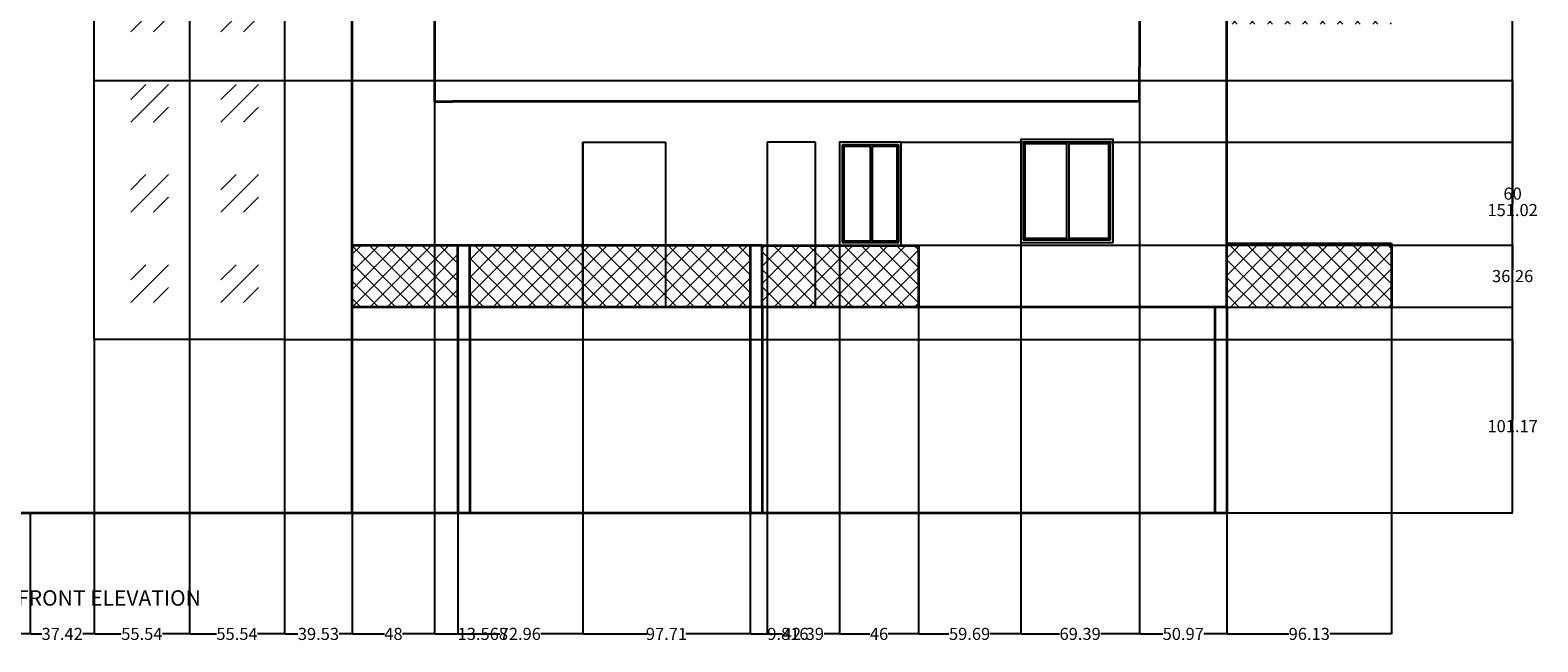
# Model space of a CAD drawing. Units: inches. Extents: x -222 to 1347, y 12 to 1073.
# Tile 3 of 4: x 467 to 1347, y 12 to 369. Entities that reach past the tile are written whole.
import ezdxf

# ---------------------------------------------------------------- set-up
doc = ezdxf.new("R2010")
doc.units = ezdxf.units.IN
doc.header["$MEASUREMENT"] = 0
for name, color, linetype, lineweight in [('A-ANNO-DIMS', 2, 'Continuous', 18), ('A-ANNO-TEXT', 7, 'Continuous', 25), ('A-DOOR', 4, 'Continuous', 25), ('A-ELEV', 7, 'Continuous', 35), ('A-ELEV-PATT', 8, 'Continuous', 13), ('A-GLAZ', 4, 'Continuous', 25)]:
    doc.layers.add(name, color=color, linetype=linetype, lineweight=lineweight)
doc.styles.get("Standard").update_dxf_attribs({"font": 'arial.ttf'})
doc.dimstyles.get("Standard").update_dxf_attribs({"dimtxt": 7.0625, "dimasz": 0.18, "dimexe": 0.18, "dimexo": 0.0625, "dimgap": 0.09, "dimtad": 0, "dimtih": 1, "dimtoh": 1, "dimdec": 4, "dimzin": 0, "dimdsep": 46, "dimlunit": 4, "dimtxsty": 'Standard', "dimcen": 0.09, "dimadec": 0, "dimazin": 0, "dimtfac": 1, "dimtdec": 4, "dimtofl": 0, "dimtmove": 0, "dimatfit": 3, "dimfxl": 1, "dimtolj": 1, "dimtzin": 0, "dimarcsym": 0})
pattern_1 = [(45, (-188.0434, -1e-13), (-5.126524, 5.126524), []), (135, (-188.0434, -1e-13), (-5.126524, -5.126524), [])]

# ---------------------------------------------------------------- blocks, each defined once
blk = doc.blocks.new('*U2')
for p, q in [((1.5, 1.5), (1.5, 58.5)), ((1.5, 58.5), (27, 58.5)), ((27, 1.5), (27, 58.5)), ((27, 58.5), (52.5, 58.5)), ((52.5, 58.5), (52.5, 1.5)), ((27, 1.5), (1.5, 1.5)), ((52.5, 1.5), (27, 1.5))]:
    blk.add_line(p, q)
blk.add_lwpolyline([(0, 0), (0, 60), (54, 60), (54, 0)], close=True)
for points in [[(26, 57.5), (26, 2.5), (2.5, 2.5), (2.5, 57.5), (26, 57.5)], [(27, 57.5), (51.5, 57.5), (51.5, 2.5), (27, 2.5)]]:
    blk.add_lwpolyline(points)
blk = doc.blocks.new('*U3')
for p, q in [((1.5, 1.5), (1.5, 58.5)), ((1.5, 58.5), (18, 58.5)), ((18, 1.5), (18, 58.5)), ((18, 58.5), (34.5, 58.5)), ((34.5, 58.5), (34.5, 1.5)), ((18, 1.5), (1.5, 1.5)), ((34.5, 1.5), (18, 1.5))]:
    blk.add_line(p, q)
blk.add_lwpolyline([(0, 0), (0, 60), (36, 60), (36, 0)], close=True)
for points in [[(17, 57.5), (17, 2.5), (2.5, 2.5), (2.5, 57.5), (17, 57.5)], [(18, 57.5), (33.5, 57.5), (33.5, 2.5), (18, 2.5)]]:
    blk.add_lwpolyline(points)
blk = doc.blocks.new('DOOR-700')
for p, q in [((0, 96.26), (0, 0)), ((0, 96.26), (23.43, 96.26)), ((23.43, 96.26), (28.14, 96.26)), ((28.14, 96.26), (28.14, 0))]:
    blk.add_line(p, q)
blk = doc.blocks.new('DOOR-1200')
for p, q in [((0, 0), (0, 96.26)), ((0, 96.26), (48.21, 96.26)), ((48.21, 96.26), (48.21, 0))]:
    blk.add_line(p, q)
blk = doc.blocks.new('*D21')
at = {"layer": 'A-ANNO-DIMS', "color": 0, "lineweight": -2, "transparency": 16777216}
for p, q in [((419.34, 327.6), (419.34, 16.83)), ((467.34, 87.6), (467.34, 16.83)), ((419.52, 17.01), (438.05, 17.01)), ((467.16, 17.01), (448.64, 17.01))]:
    blk.add_line(p, q, dxfattribs=at)
at = {"layer": 'A-ANNO-DIMS', "color": 0, "transparency": 16777216}
for points in [[(419.52, 17.04), (419.52, 16.98), (419.34, 17.01)], [(467.16, 17.04), (467.16, 16.98), (467.34, 17.01)]]:
    blk.add_solid(points, dxfattribs=at)
at = {"layer": 'Defpoints', "color": 0, "transparency": 16777216}
for p in [(419.34, 327.66), (467.34, 87.66), (467.34, 17.01)]:
    blk.add_point(p, dxfattribs=at)
at = {"layer": 'A-ANNO-DIMS', "color": 0, "transparency": 16777216, "insert": (443.34, 17.01), "char_height": 7.062, "attachment_point": 5}
blk.add_mtext('\\A1;48', dxfattribs=at)
blk = doc.blocks.new('*D22')
at = {"layer": 'A-ANNO-DIMS', "color": 0, "lineweight": -2, "transparency": 16777216}
for p, q in [((504.77, 188.77), (504.77, 16.83)), ((467.34, 87.6), (467.34, 16.83)), ((467.52, 17.01), (474.09, 17.01)), ((504.59, 17.01), (498.02, 17.01))]:
    blk.add_line(p, q, dxfattribs=at)
at = {"layer": 'A-ANNO-DIMS', "color": 0, "transparency": 16777216}
for points in [[(467.52, 17.04), (467.52, 16.98), (467.34, 17.01)], [(504.59, 17.04), (504.59, 16.98), (504.77, 17.01)]]:
    blk.add_solid(points, dxfattribs=at)
at = {"layer": 'Defpoints', "color": 0, "transparency": 16777216}
for p in [(504.77, 188.83), (467.34, 87.66), (504.77, 17.01)]:
    blk.add_point(p, dxfattribs=at)
at = {"layer": 'A-ANNO-DIMS', "color": 0, "transparency": 16777216, "insert": (486.05, 17.01), "char_height": 7.062, "attachment_point": 5}
blk.add_mtext('\\A1;37.42', dxfattribs=at)
blk = doc.blocks.new('*D23')
at = {"layer": 'A-ANNO-DIMS', "color": 0, "lineweight": -2, "transparency": 16777216}
for p, q in [((504.77, 188.77), (504.77, 16.83)), ((560.31, 188.77), (560.31, 16.83)), ((504.95, 17.01), (520.55, 17.01)), ((560.13, 17.01), (544.53, 17.01))]:
    blk.add_line(p, q, dxfattribs=at)
at = {"layer": 'A-ANNO-DIMS', "color": 0, "transparency": 16777216}
for points in [[(504.95, 17.04), (504.95, 16.98), (504.77, 17.01)], [(560.13, 17.04), (560.13, 16.98), (560.31, 17.01)]]:
    blk.add_solid(points, dxfattribs=at)
at = {"layer": 'Defpoints', "color": 0, "transparency": 16777216}
for p in [(504.77, 188.83), (560.31, 188.83), (560.31, 17.01)]:
    blk.add_point(p, dxfattribs=at)
at = {"layer": 'A-ANNO-DIMS', "color": 0, "transparency": 16777216, "insert": (532.54, 17.01), "char_height": 7.062, "attachment_point": 5}
blk.add_mtext('\\A1;55.54', dxfattribs=at)
blk = doc.blocks.new('*D24')
at = {"layer": 'A-ANNO-DIMS', "color": 0, "lineweight": -2, "transparency": 16777216}
for p, q in [((560.31, 188.77), (560.31, 16.83)), ((615.85, 188.77), (615.85, 16.83)), ((560.49, 17.01), (576.09, 17.01)), ((615.67, 17.01), (600.07, 17.01))]:
    blk.add_line(p, q, dxfattribs=at)
at = {"layer": 'A-ANNO-DIMS', "color": 0, "transparency": 16777216}
for points in [[(560.49, 17.04), (560.49, 16.98), (560.31, 17.01)], [(615.67, 17.04), (615.67, 16.98), (615.85, 17.01)]]:
    blk.add_solid(points, dxfattribs=at)
at = {"layer": 'Defpoints', "color": 0, "transparency": 16777216}
for p in [(560.31, 188.83), (615.85, 188.83), (615.85, 17.01)]:
    blk.add_point(p, dxfattribs=at)
at = {"layer": 'A-ANNO-DIMS', "color": 0, "transparency": 16777216, "insert": (588.08, 17.01), "char_height": 7.062, "attachment_point": 5}
blk.add_mtext('\\A1;55.54', dxfattribs=at)
blk = doc.blocks.new('*D25')
at = {"layer": 'A-ANNO-DIMS', "color": 0, "lineweight": -2, "transparency": 16777216}
for p, q in [((615.85, 188.77), (615.85, 16.83)), ((655.39, 87.6), (655.39, 16.83)), ((616.03, 17.01), (623.62, 17.01)), ((655.21, 17.01), (647.62, 17.01))]:
    blk.add_line(p, q, dxfattribs=at)
at = {"layer": 'A-ANNO-DIMS', "color": 0, "transparency": 16777216}
for points in [[(616.03, 17.04), (616.03, 16.98), (615.85, 17.01)], [(655.21, 17.04), (655.21, 16.98), (655.39, 17.01)]]:
    blk.add_solid(points, dxfattribs=at)
at = {"layer": 'Defpoints', "color": 0, "transparency": 16777216}
for p in [(615.85, 188.83), (655.39, 87.66), (655.39, 17.01)]:
    blk.add_point(p, dxfattribs=at)
at = {"layer": 'A-ANNO-DIMS', "color": 0, "transparency": 16777216, "insert": (635.62, 17.01), "char_height": 7.062, "attachment_point": 5}
blk.add_mtext('\\A1;39.53', dxfattribs=at)
blk = doc.blocks.new('*D26')
at = {"layer": 'A-ANNO-DIMS', "color": 0, "lineweight": -2, "transparency": 16777216}
for p, q in [((703.39, 327.6), (703.39, 16.83)), ((655.39, 87.6), (655.39, 16.83)), ((655.57, 17.01), (674.09, 17.01)), ((703.21, 17.01), (684.68, 17.01))]:
    blk.add_line(p, q, dxfattribs=at)
at = {"layer": 'A-ANNO-DIMS', "color": 0, "transparency": 16777216}
for points in [[(655.57, 17.04), (655.57, 16.98), (655.39, 17.01)], [(703.21, 17.04), (703.21, 16.98), (703.39, 17.01)]]:
    blk.add_solid(points, dxfattribs=at)
at = {"layer": 'Defpoints', "color": 0, "transparency": 16777216}
for p in [(703.39, 327.66), (655.39, 87.66), (703.39, 17.01)]:
    blk.add_point(p, dxfattribs=at)
at = {"layer": 'A-ANNO-DIMS', "color": 0, "transparency": 16777216, "insert": (679.39, 17.01), "char_height": 7.062, "attachment_point": 5}
blk.add_mtext('\\A1;48', dxfattribs=at)
blk = doc.blocks.new('*D27')
at = {"layer": 'A-ANNO-DIMS', "color": 0, "lineweight": -2, "transparency": 16777216}
for p, q in [((703.39, 327.6), (703.39, 16.83)), ((716.95, 87.6), (716.95, 16.83)), ((703.57, 17.01), (716.77, 17.01)), ((716.95, 17.01), (717.13, 17.01))]:
    blk.add_line(p, q, dxfattribs=at)
at = {"layer": 'A-ANNO-DIMS', "color": 0, "transparency": 16777216}
for points in [[(703.57, 17.04), (703.57, 16.98), (703.39, 17.01)], [(716.77, 17.04), (716.77, 16.98), (716.95, 17.01)]]:
    blk.add_solid(points, dxfattribs=at)
at = {"layer": 'Defpoints', "color": 0, "transparency": 16777216}
for p in [(703.39, 327.66), (716.95, 87.66), (716.95, 17.01)]:
    blk.add_point(p, dxfattribs=at)
at = {"layer": 'A-ANNO-DIMS', "color": 0, "transparency": 16777216, "insert": (731.56, 17.01), "char_height": 7.062, "attachment_point": 5}
blk.add_mtext('\\A1;13.568', dxfattribs=at)
blk = doc.blocks.new('*D28')
at = {"layer": 'A-ANNO-DIMS', "color": 0, "lineweight": -2, "transparency": 16777216}
for p, q in [((789.92, 303.86), (789.92, 16.83)), ((716.95, 87.6), (716.95, 16.83)), ((717.13, 17.01), (741.46, 17.01)), ((789.74, 17.01), (765.41, 17.01))]:
    blk.add_line(p, q, dxfattribs=at)
at = {"layer": 'A-ANNO-DIMS', "color": 0, "transparency": 16777216}
for points in [[(717.13, 17.04), (717.13, 16.98), (716.95, 17.01)], [(789.74, 17.04), (789.74, 16.98), (789.92, 17.01)]]:
    blk.add_solid(points, dxfattribs=at)
at = {"layer": 'Defpoints', "color": 0, "transparency": 16777216}
for p in [(789.92, 303.93), (716.95, 87.66), (789.92, 17.01)]:
    blk.add_point(p, dxfattribs=at)
at = {"layer": 'A-ANNO-DIMS', "color": 0, "transparency": 16777216, "insert": (753.44, 17.01), "char_height": 7.062, "attachment_point": 5}
blk.add_mtext('\\A1;72.96', dxfattribs=at)
blk = doc.blocks.new('*D29')
at = {"layer": 'A-ANNO-DIMS', "color": 0, "lineweight": -2, "transparency": 16777216}
for p, q in [((789.92, 303.86), (789.92, 16.83)), ((887.63, 87.6), (887.63, 16.83)), ((790.1, 17.01), (827.45, 17.01)), ((887.45, 17.01), (850.1, 17.01))]:
    blk.add_line(p, q, dxfattribs=at)
at = {"layer": 'A-ANNO-DIMS', "color": 0, "transparency": 16777216}
for points in [[(790.1, 17.04), (790.1, 16.98), (789.92, 17.01)], [(887.45, 17.04), (887.45, 16.98), (887.63, 17.01)]]:
    blk.add_solid(points, dxfattribs=at)
at = {"layer": 'Defpoints', "color": 0, "transparency": 16777216}
for p in [(789.92, 303.93), (887.63, 87.66), (887.63, 17.01)]:
    blk.add_point(p, dxfattribs=at)
at = {"layer": 'A-ANNO-DIMS', "color": 0, "transparency": 16777216, "insert": (838.77, 17.01), "char_height": 7.062, "attachment_point": 5}
blk.add_mtext('\\A1;97.71', dxfattribs=at)
blk = doc.blocks.new('*D30')
at = {"layer": 'A-ANNO-DIMS', "color": 0, "lineweight": -2, "transparency": 16777216}
for p, q in [((897.45, 303.86), (897.45, 16.83)), ((887.63, 87.6), (887.63, 16.83)), ((887.81, 17.01), (897.27, 17.01)), ((897.45, 17.01), (897.63, 17.01))]:
    blk.add_line(p, q, dxfattribs=at)
at = {"layer": 'A-ANNO-DIMS', "color": 0, "transparency": 16777216}
for points in [[(887.81, 17.04), (887.81, 16.98), (887.63, 17.01)], [(897.27, 17.04), (897.27, 16.98), (897.45, 17.01)]]:
    blk.add_solid(points, dxfattribs=at)
at = {"layer": 'Defpoints', "color": 0, "transparency": 16777216}
for p in [(897.45, 303.93), (887.63, 87.66), (897.45, 17.01)]:
    blk.add_point(p, dxfattribs=at)
at = {"layer": 'A-ANNO-DIMS', "color": 0, "transparency": 16777216, "insert": (909.63, 17.01), "char_height": 7.062, "attachment_point": 5}
blk.add_mtext('\\A1;9.816', dxfattribs=at)
blk = doc.blocks.new('*D31')
at = {"layer": 'A-ANNO-DIMS', "color": 0, "lineweight": -2, "transparency": 16777216}
for p, q in [((897.45, 303.86), (897.45, 16.83)), ((939.84, 243.86), (939.84, 16.83)), ((897.63, 17.01), (906.49, 17.01)), ((939.66, 17.01), (930.8, 17.01))]:
    blk.add_line(p, q, dxfattribs=at)
at = {"layer": 'A-ANNO-DIMS', "color": 0, "transparency": 16777216}
for points in [[(897.63, 17.04), (897.63, 16.98), (897.45, 17.01)], [(939.66, 17.04), (939.66, 16.98), (939.84, 17.01)]]:
    blk.add_solid(points, dxfattribs=at)
at = {"layer": 'Defpoints', "color": 0, "transparency": 16777216}
for p in [(897.45, 303.93), (939.84, 243.93), (939.84, 17.01)]:
    blk.add_point(p, dxfattribs=at)
at = {"layer": 'A-ANNO-DIMS', "color": 0, "transparency": 16777216, "insert": (918.64, 17.01), "char_height": 7.062, "attachment_point": 5}
blk.add_mtext('\\A1;42.39', dxfattribs=at)
blk = doc.blocks.new('*D32')
at = {"layer": 'A-ANNO-DIMS', "color": 0, "lineweight": -2, "transparency": 16777216}
for p, q in [((939.84, 243.86), (939.84, 16.83)), ((985.84, 207.6), (985.84, 16.83)), ((940.02, 17.01), (957.55, 17.01)), ((985.66, 17.01), (968.13, 17.01))]:
    blk.add_line(p, q, dxfattribs=at)
at = {"layer": 'A-ANNO-DIMS', "color": 0, "transparency": 16777216}
for points in [[(940.02, 17.04), (940.02, 16.98), (939.84, 17.01)], [(985.66, 17.04), (985.66, 16.98), (985.84, 17.01)]]:
    blk.add_solid(points, dxfattribs=at)
at = {"layer": 'Defpoints', "color": 0, "transparency": 16777216}
for p in [(939.84, 243.93), (985.84, 207.66), (985.84, 17.01)]:
    blk.add_point(p, dxfattribs=at)
at = {"layer": 'A-ANNO-DIMS', "color": 0, "transparency": 16777216, "insert": (962.84, 17.01), "char_height": 7.062, "attachment_point": 5}
blk.add_mtext('\\A1;46', dxfattribs=at)
blk = doc.blocks.new('*D33')
at = {"layer": 'A-ANNO-DIMS', "color": 0, "lineweight": -2, "transparency": 16777216}
for p, q in [((1045.53, 245.36), (1045.53, 16.83)), ((985.84, 207.6), (985.84, 16.83)), ((986.02, 17.01), (1003.67, 17.01)), ((1045.35, 17.01), (1027.7, 17.01))]:
    blk.add_line(p, q, dxfattribs=at)
at = {"layer": 'A-ANNO-DIMS', "color": 0, "transparency": 16777216}
for points in [[(986.02, 17.04), (986.02, 16.98), (985.84, 17.01)], [(1045.35, 17.04), (1045.35, 16.98), (1045.53, 17.01)]]:
    blk.add_solid(points, dxfattribs=at)
at = {"layer": 'Defpoints', "color": 0, "transparency": 16777216}
for p in [(1045.53, 245.43), (985.84, 207.66), (1045.53, 17.01)]:
    blk.add_point(p, dxfattribs=at)
at = {"layer": 'A-ANNO-DIMS', "color": 0, "transparency": 16777216, "insert": (1015.69, 17.01), "char_height": 7.062, "attachment_point": 5}
blk.add_mtext('\\A1;59.69', dxfattribs=at)
blk = doc.blocks.new('*D34')
at = {"layer": 'A-ANNO-DIMS', "color": 0, "lineweight": -2, "transparency": 16777216}
for p, q in [((1114.92, 327.6), (1114.92, 16.83)), ((1045.53, 245.36), (1045.53, 16.83)), ((1045.71, 17.01), (1068.2, 17.01)), ((1114.74, 17.01), (1092.26, 17.01))]:
    blk.add_line(p, q, dxfattribs=at)
at = {"layer": 'A-ANNO-DIMS', "color": 0, "transparency": 16777216}
for points in [[(1045.71, 17.04), (1045.71, 16.98), (1045.53, 17.01)], [(1114.74, 17.04), (1114.74, 16.98), (1114.92, 17.01)]]:
    blk.add_solid(points, dxfattribs=at)
at = {"layer": 'Defpoints', "color": 0, "transparency": 16777216}
for p in [(1114.92, 327.66), (1045.53, 245.43), (1114.92, 17.01)]:
    blk.add_point(p, dxfattribs=at)
at = {"layer": 'A-ANNO-DIMS', "color": 0, "transparency": 16777216, "insert": (1080.23, 17.01), "char_height": 7.062, "attachment_point": 5}
blk.add_mtext('\\A1;69.39', dxfattribs=at)
blk = doc.blocks.new('*D35')
at = {"layer": 'A-ANNO-DIMS', "color": 0, "lineweight": -2, "transparency": 16777216}
for p, q in [((1114.92, 327.6), (1114.92, 16.83)), ((1165.89, 87.6), (1165.89, 16.83)), ((1115.1, 17.01), (1128.4, 17.01)), ((1165.71, 17.01), (1152.41, 17.01))]:
    blk.add_line(p, q, dxfattribs=at)
at = {"layer": 'A-ANNO-DIMS', "color": 0, "transparency": 16777216}
for points in [[(1115.1, 17.04), (1115.1, 16.98), (1114.92, 17.01)], [(1165.71, 17.04), (1165.71, 16.98), (1165.89, 17.01)]]:
    blk.add_solid(points, dxfattribs=at)
at = {"layer": 'Defpoints', "color": 0, "transparency": 16777216}
for p in [(1114.92, 327.66), (1165.89, 87.66), (1165.89, 17.01)]:
    blk.add_point(p, dxfattribs=at)
at = {"layer": 'A-ANNO-DIMS', "color": 0, "transparency": 16777216, "insert": (1140.41, 17.01), "char_height": 7.062, "attachment_point": 5}
blk.add_mtext('\\A1;50.97', dxfattribs=at)
blk = doc.blocks.new('*D36')
at = {"layer": 'A-ANNO-DIMS', "color": 0, "lineweight": -2, "transparency": 16777216}
for p, q in [((1262.02, 207.6), (1262.02, 16.83)), ((1165.89, 87.6), (1165.89, 16.83)), ((1166.07, 17.01), (1201.95, 17.01)), ((1261.84, 17.01), (1225.96, 17.01))]:
    blk.add_line(p, q, dxfattribs=at)
at = {"layer": 'A-ANNO-DIMS', "color": 0, "transparency": 16777216}
for points in [[(1166.07, 17.04), (1166.07, 16.98), (1165.89, 17.01)], [(1261.84, 17.04), (1261.84, 16.98), (1262.02, 17.01)]]:
    blk.add_solid(points, dxfattribs=at)
at = {"layer": 'Defpoints', "color": 0, "transparency": 16777216}
for p in [(1262.02, 207.66), (1165.89, 87.66), (1262.02, 17.01)]:
    blk.add_point(p, dxfattribs=at)
at = {"layer": 'A-ANNO-DIMS', "color": 0, "transparency": 16777216, "insert": (1213.96, 17.01), "char_height": 7.062, "attachment_point": 5}
blk.add_mtext('\\A1;96.13', dxfattribs=at)
blk = doc.blocks.new('*D37')
at = {"layer": 'A-ANNO-DIMS', "color": 0, "lineweight": -2, "transparency": 16777216}
for p, q in [((655.45, 997.49), (1332.85, 997.49)), ((1332.67, 997.31), (1332.67, 546.27)), ((1332.67, 87.84), (1332.67, 538.88)), ((655.45, 87.66), (1332.85, 87.66))]:
    blk.add_line(p, q, dxfattribs=at)
at = {"layer": 'A-ANNO-DIMS', "color": 0, "transparency": 16777216}
for points in [[(1332.64, 997.31), (1332.7, 997.31), (1332.67, 997.49)], [(1332.64, 87.84), (1332.7, 87.84), (1332.67, 87.66)]]:
    blk.add_solid(points, dxfattribs=at)
at = {"layer": 'Defpoints', "color": 0, "transparency": 16777216}
for p in [(655.39, 997.49), (1332.67, 997.49), (655.39, 87.66)]:
    blk.add_point(p, dxfattribs=at)
at = {"layer": 'A-ANNO-DIMS', "color": 0, "transparency": 16777216, "insert": (1332.67, 542.58), "char_height": 7.062, "attachment_point": 5}
blk.add_mtext('\\A1;909.8', dxfattribs=at)
blk = doc.blocks.new('*D60')
at = {"layer": 'A-ANNO-DIMS', "color": 0, "lineweight": -2, "transparency": 16777216}
for p, q in [((975.9, 243.93), (1332.85, 243.93)), ((1332.67, 243.75), (1332.67, 229.49)), ((1332.67, 207.84), (1332.67, 222.1)), ((985.9, 207.66), (1332.85, 207.66))]:
    blk.add_line(p, q, dxfattribs=at)
at = {"layer": 'A-ANNO-DIMS', "color": 0, "transparency": 16777216}
for points in [[(1332.64, 243.75), (1332.7, 243.75), (1332.67, 243.93)], [(1332.64, 207.84), (1332.7, 207.84), (1332.67, 207.66)]]:
    blk.add_solid(points, dxfattribs=at)
at = {"layer": 'Defpoints', "color": 0, "transparency": 16777216}
for p in [(975.84, 243.93), (1332.67, 243.93), (985.84, 207.66)]:
    blk.add_point(p, dxfattribs=at)
at = {"layer": 'A-ANNO-DIMS', "color": 0, "transparency": 16777216, "insert": (1332.67, 225.8), "char_height": 7.062, "attachment_point": 5}
blk.add_mtext('\\A1;36.26', dxfattribs=at)
blk = doc.blocks.new('*D61')
at = {"layer": 'A-ANNO-DIMS', "color": 0, "lineweight": -2, "transparency": 16777216}
for p, q in [((975.9, 303.93), (1332.85, 303.93)), ((1332.67, 303.75), (1332.67, 277.62)), ((1332.67, 244.11), (1332.67, 270.23)), ((975.9, 243.93), (1332.85, 243.93))]:
    blk.add_line(p, q, dxfattribs=at)
at = {"layer": 'A-ANNO-DIMS', "color": 0, "transparency": 16777216}
for points in [[(1332.64, 303.75), (1332.7, 303.75), (1332.67, 303.93)], [(1332.64, 244.11), (1332.7, 244.11), (1332.67, 243.93)]]:
    blk.add_solid(points, dxfattribs=at)
at = {"layer": 'Defpoints', "color": 0, "transparency": 16777216}
for p in [(975.84, 303.93), (1332.67, 303.93), (975.84, 243.93)]:
    blk.add_point(p, dxfattribs=at)
at = {"layer": 'A-ANNO-DIMS', "color": 0, "transparency": 16777216, "insert": (1332.67, 273.93), "char_height": 7.062, "attachment_point": 5}
blk.add_mtext('\\A1;60', dxfattribs=at)
blk = doc.blocks.new('*D70')
at = {"layer": 'A-ANNO-DIMS', "color": 0, "lineweight": -2, "transparency": 16777216}
for p, q in [((615.92, 188.83), (1332.85, 188.83)), ((1332.67, 188.65), (1332.67, 141.95)), ((1332.67, 87.84), (1332.67, 134.55)), ((467.41, 87.66), (1332.85, 87.66))]:
    blk.add_line(p, q, dxfattribs=at)
at = {"layer": 'A-ANNO-DIMS', "color": 0, "transparency": 16777216}
for points in [[(1332.64, 188.65), (1332.7, 188.65), (1332.67, 188.83)], [(1332.64, 87.84), (1332.7, 87.84), (1332.67, 87.66)]]:
    blk.add_solid(points, dxfattribs=at)
at = {"layer": 'Defpoints', "color": 0, "transparency": 16777216}
for p in [(615.85, 188.83), (1332.67, 188.83), (467.34, 87.66)]:
    blk.add_point(p, dxfattribs=at)
at = {"layer": 'A-ANNO-DIMS', "color": 0, "transparency": 16777216, "insert": (1332.67, 138.25), "char_height": 7.062, "attachment_point": 5}
blk.add_mtext('\\A1;101.17', dxfattribs=at)
blk = doc.blocks.new('*D71')
at = {"layer": 'A-ANNO-DIMS', "color": 0, "lineweight": -2, "transparency": 16777216}
for p, q in [((615.92, 339.85), (1332.85, 339.85)), ((1332.67, 339.67), (1332.67, 268.04)), ((1332.67, 189.01), (1332.67, 260.65)), ((615.92, 188.83), (1332.85, 188.83))]:
    blk.add_line(p, q, dxfattribs=at)
at = {"layer": 'A-ANNO-DIMS', "color": 0, "transparency": 16777216}
for points in [[(1332.64, 339.67), (1332.7, 339.67), (1332.67, 339.85)], [(1332.64, 189.01), (1332.7, 189.01), (1332.67, 188.83)]]:
    blk.add_solid(points, dxfattribs=at)
at = {"layer": 'Defpoints', "color": 0, "transparency": 16777216}
for p in [(615.85, 339.85), (1332.67, 339.85), (615.85, 188.83)]:
    blk.add_point(p, dxfattribs=at)
at = {"layer": 'A-ANNO-DIMS', "color": 0, "transparency": 16777216, "insert": (1332.67, 264.34), "char_height": 7.062, "attachment_point": 5}
blk.add_mtext('\\A1;151.02', dxfattribs=at)
blk = doc.blocks.new('*D72')
at = {"layer": 'A-ANNO-DIMS', "color": 0, "lineweight": -2, "transparency": 16777216}
for p, q in [((615.92, 492.24), (1332.85, 492.24)), ((1332.67, 492.06), (1332.67, 419.74)), ((1332.67, 340.03), (1332.67, 412.35)), ((615.92, 339.85), (1332.85, 339.85))]:
    blk.add_line(p, q, dxfattribs=at)
at = {"layer": 'A-ANNO-DIMS', "color": 0, "transparency": 16777216}
for points in [[(1332.64, 492.06), (1332.7, 492.06), (1332.67, 492.24)], [(1332.64, 340.03), (1332.7, 340.03), (1332.67, 339.85)]]:
    blk.add_solid(points, dxfattribs=at)
at = {"layer": 'Defpoints', "color": 0, "transparency": 16777216}
for p in [(615.85, 492.24), (1332.67, 492.24), (615.85, 339.85)]:
    blk.add_point(p, dxfattribs=at)
at = {"layer": 'A-ANNO-DIMS', "color": 0, "transparency": 16777216, "insert": (1332.67, 416.05), "char_height": 7.062, "attachment_point": 5}
blk.add_mtext('\\A1;152.4', dxfattribs=at)

msp = doc.modelspace()

# ---------------------------------------------------------------- hatches: boundary and pattern name
at = {"layer": 'A-ELEV-PATT'}
h = msp.add_hatch(dxfattribs=at)
h.set_pattern_fill('GOST_GLASS', color=256, scale=6.2)
h.set_pattern_definition([(45, (0, 0), (52.6087, 0), [31, -43.4]), (45, (13.152, 0), (52.6087, 0), [12.4, -62]), (45, (0, 13.152), (52.6087, 0), [12.4, -62])])
h.paths.add_polyline_path([(560.3092, 856.413), (504.7654, 856.413), (504.7654, 643.1444), (560.3092, 643.1444)])
h.paths.add_polyline_path([(615.8531, 856.413), (560.3092, 856.413), (560.3092, 643.1444), (615.8531, 643.1444)])
h.paths.add_polyline_path([(560.3092, 643.1444), (504.7654, 643.1444), (504.7654, 492.2448), (560.3092, 492.2448)])
h.paths.add_polyline_path([(615.8531, 643.1444), (560.3092, 643.1444), (560.3092, 492.2448), (615.8531, 492.2448)])
h.paths.add_polyline_path([(560.3092, 492.2448), (504.7654, 492.2448), (504.7654, 339.8505), (560.3092, 339.8505)])
h.paths.add_polyline_path([(615.8531, 492.2448), (560.3092, 492.2448), (560.3092, 339.8505), (615.8531, 339.8505)])
h.paths.add_polyline_path([(560.3092, 339.8505), (504.7654, 339.8505), (504.7654, 188.834), (560.3092, 188.834)])
h.paths.add_polyline_path([(615.8531, 339.8505), (560.3092, 339.8505), (560.3092, 188.834), (615.8531, 188.834)])
h = msp.add_hatch(dxfattribs=at)
h.set_pattern_fill('ANSI37', color=256, scale=58)
h.set_pattern_definition(pattern_1)
h.paths.add_polyline_path([(1165.8907, 648.7576), (1262.0222, 648.7576), (1262.0222, 630.2077), (1165.8907, 630.2077)])
h.paths.add_polyline_path([(1165.8907, 630.2077), (1262.0222, 630.2077), (1262.0222, 611.6578), (1165.8907, 611.6578)])
h.paths.add_polyline_path([(1165.8907, 529.8651), (1262.0222, 529.8651), (1262.0222, 511.3152), (1165.8907, 511.3152)])
h.paths.add_polyline_path([(1165.8907, 511.3152), (1262.0222, 511.3152), (1262.0222, 492.7653), (1165.8907, 492.7653)])
h.paths.add_polyline_path([(1165.8907, 409.8651), (1262.0222, 409.8651), (1262.0222, 391.3152), (1165.8907, 391.3152)])
h.paths.add_polyline_path([(1165.8907, 391.3152), (1262.0222, 391.3152), (1262.0222, 372.7653), (1165.8907, 372.7653)])
h.paths.add_polyline_path([(1165.8907, 244.764), (1262.0222, 244.764), (1262.0222, 226.2141), (1165.8907, 226.2141)])
h.paths.add_polyline_path([(1165.8907, 226.2141), (1262.0222, 226.2141), (1262.0222, 207.6642), (1165.8907, 207.6642)])
h = msp.add_hatch(dxfattribs=at)
h.set_pattern_fill('ANSI37', color=256, scale=58)
h.set_pattern_definition(pattern_1)
h.paths.add_polyline_path([(925.5902, 243.6642), (985.8399, 243.6642), (985.8399, 225.6642), (925.5902, 225.6642)])
h.paths.add_polyline_path([(925.5902, 225.6642), (985.8399, 225.6642), (985.8399, 207.6642), (925.5902, 207.6642)])
h.paths.add_polyline_path([(897.4464, 243.6642), (925.5902, 243.6642), (925.5902, 225.6642), (897.4464, 225.6642)])
h.paths.add_polyline_path([(897.4464, 225.6642), (925.5902, 225.6642), (925.5902, 207.6642), (897.4464, 207.6642)])
h.paths.add_polyline_path([(894.63, 243.6642), (897.4464, 243.6642), (897.4464, 225.6642), (894.63, 225.6642)])
h.paths.add_polyline_path([(894.63, 225.6642), (897.4464, 225.6642), (897.4464, 207.6642), (894.63, 207.6642)])
h.paths.add_polyline_path([(838.1288, 243.6642), (887.63, 243.6642), (887.63, 225.6642), (838.1288, 225.6642)])
h.paths.add_polyline_path([(838.1288, 225.6642), (887.63, 225.6642), (887.63, 207.6642), (838.1288, 207.6642)])
h.paths.add_polyline_path([(789.9158, 243.6642), (838.1288, 243.6642), (838.1288, 225.6642), (789.9158, 225.6642)])
h.paths.add_polyline_path([(789.9158, 225.6642), (838.1288, 225.6642), (838.1288, 207.6642), (789.9158, 207.6642)])
h.paths.add_polyline_path([(723.9547, 243.6642), (789.9158, 243.6642), (789.9158, 225.6642), (723.9547, 225.6642)])
h.paths.add_polyline_path([(723.9547, 225.6642), (789.9158, 225.6642), (789.9158, 207.6642), (723.9547, 207.6642)])
h.paths.add_polyline_path([(655.387, 243.6642), (716.9547, 243.6642), (716.9547, 225.6642), (655.387, 225.6642)])
h.paths.add_polyline_path([(655.387, 225.6642), (716.9547, 225.6642), (716.9547, 207.6642), (655.387, 207.6642)])

# ---------------------------------------------------------------- linework, layer by layer
at = {"layer": 'A-ELEV'}
for p, q in [((655.387, 87.6642), (655.387, 997.488)), ((1165.8907, 207.6642), (1165.8907, 780.7653)), ((1114.924, 584.7569), (1114.924, 347.9663)), ((703.387, 447.6642), (703.387, 327.6642)), ((1114.924, 327.6642), (1114.924, 347.9663)), ((703.387, 327.6642), (713.9581, 327.6642)), ((1114.924, 327.6642), (713.9581, 327.6642)), ((723.9547, 243.6642), (655.387, 243.6642)), ((716.9547, 207.6642), (716.9547, 243.6642)), ((887.63, 243.6642), (723.9547, 243.6642)), ((723.9547, 207.6642), (723.9547, 243.6642)), ((894.63, 243.6642), (887.63, 243.6642)), ((887.63, 243.6642), (887.63, 207.6642)), ((894.63, 207.6642), (894.63, 243.6642)), ((894.63, 243.6642), (985.8399, 243.6642)), ((985.8399, 243.6642), (985.8399, 207.6642)), ((1165.8907, 244.764), (1262.0222, 244.764)), ((1262.0222, 244.764), (1262.0222, 207.6642)), ((1165.8907, 207.6642), (655.387, 207.6642)), ((716.9547, 207.6642), (716.9547, 87.6642)), ((723.9547, 207.6642), (723.9547, 87.6642)), ((887.63, 207.6642), (887.63, 87.6642)), ((894.63, 207.6642), (894.63, 87.6642)), ((1158.8907, 207.6642), (1158.8907, 87.6642)), ((1165.8907, 207.6642), (1165.8907, 87.6642)), ((40.3442, 87.6642), (971.5102, 87.6642)), ((971.5102, 87.6642), (1165.8907, 87.6642))]:
    msp.add_line(p, q, dxfattribs=at)
at = {"layer": 'A-GLAZ'}
for p, q in [((560.3092, 856.413), (560.3092, 188.834)), ((504.7654, 339.8505), (615.8531, 339.8505))]:
    msp.add_line(p, q, dxfattribs=at)
msp.add_lwpolyline([(504.7654, 856.413), (615.8531, 856.413), (615.8531, 188.834), (504.7654, 188.834)], close=True, dxfattribs=at)

# ---------------------------------------------------------------- block references
at = {"layer": 'A-DOOR'}
msp.add_blockref('DOOR-1200', (789.9161, 207.664), dxfattribs=at)
at = {"layer": 'A-DOOR', "extrusion": (0, 0, -1), "zscale": -1}
msp.add_blockref('DOOR-700', (-925.5906, 207.664), dxfattribs=at)
at = {"layer": 'A-GLAZ', "xscale": -1}
for name, p in [('*U3', (975.8393, 243.9265)), ('*U2', (1099.5315, 245.4265))]:
    msp.add_blockref(name, p, dxfattribs=at)

# ---------------------------------------------------------------- texts
at = {"layer": 'A-ANNO-TEXT', "insert": (459.7334, 42.4682), "char_height": 9, "attachment_point": 1}
msp.add_mtext_dynamic_manual_height_columns('FRONT ELEVATION', width=262.403547, gutter_width=1, heights=[0], dxfattribs=at)

# ---------------------------------------------------------------- dimensions: what is measured, and where the dimension line sits
at = {"layer": 'A-ANNO-DIMS'}
for base, p1, p2, override, picture, middle in [((1332.6722, 997.488), (655.387, 87.6642), (655.387, 997.488), {"dimdec": 1, "dimlfac": 1, "dimrnd": 0, "dimzin": 0, "dimdsep": 46, "dimlunit": 2}, '*D37', (1332.6722, 542.5761)), ((1332.6722, 492.2448), (615.8531, 339.8505), (615.8531, 492.2448), {"dimdec": 1, "dimlfac": 1, "dimrnd": 0, "dimzin": 0, "dimdsep": 46, "dimlunit": 2}, '*D72', (1332.6722, 416.0477)), ((1332.6722, 339.8505), (615.8531, 188.834), (615.8531, 339.8505), {"dimdec": 2, "dimlfac": 1, "dimrnd": 0, "dimzin": 0, "dimdsep": 46, "dimlunit": 2}, '*D71', (1332.6722, 264.3423)), ((1332.6722, 303.9265), (975.8393, 243.9265), (975.8393, 303.9265), {"dimdec": 0, "dimlfac": 1, "dimrnd": 0, "dimzin": 0, "dimdsep": 46, "dimlunit": 2}, '*D61', (1332.6722, 273.9265)), ((1332.6722, 243.9265), (985.8399, 207.6642), (975.8393, 243.9265), {"dimdec": 2, "dimlfac": 1, "dimrnd": 0, "dimzin": 0, "dimdsep": 46, "dimlunit": 2}, '*D60', (1332.6722, 225.7953)), ((1332.6722, 188.834), (467.3436, 87.6642), (615.8531, 188.834), {"dimdec": 2, "dimlfac": 1, "dimrnd": 0, "dimzin": 0, "dimdsep": 46, "dimlunit": 2}, '*D70', (1332.6722, 138.2491))]:
    dim = msp.add_linear_dim(base=base, p1=p1, p2=p2, angle=90, dimstyle='Standard', override=override, dxfattribs=at)
    dim.commit()
    dim.dimension.update_dxf_attribs({"geometry": picture, "text_midpoint": middle})
for base, p1, p2, override, picture, middle in [((467.3436, 17.0142), (419.3436, 327.6642), (467.3436, 87.6642), {"dimdec": 0, "dimlfac": 1, "dimrnd": 0, "dimzin": 0, "dimdsep": 46, "dimlunit": 2}, '*D21', (443.3436, 17.0142)), ((703.387, 17.0142), (655.387, 87.6642), (703.387, 327.6642), {"dimdec": 0, "dimlfac": 1, "dimrnd": 0, "dimzin": 0, "dimdsep": 46, "dimlunit": 2}, '*D26', (679.387, 17.0142)), ((716.9547, 17.0142), (703.387, 327.6642), (716.9547, 87.6642), {"dimdec": 3, "dimlfac": 1, "dimrnd": 0, "dimzin": 0, "dimdsep": 46, "dimlunit": 2}, '*D27', (731.5592, 17.0142)), ((1114.924, 17.0142), (1045.5315, 245.4265), (1114.924, 327.6642), {"dimdec": 2, "dimlfac": 1, "dimrnd": 0, "dimzin": 0, "dimdsep": 46, "dimlunit": 2}, '*D34', (1080.2278, 17.0142)), ((1165.8907, 17.0142), (1114.924, 327.6642), (1165.8907, 87.6642), {"dimdec": 2, "dimlfac": 1, "dimrnd": 0, "dimzin": 0, "dimdsep": 46, "dimlunit": 2}, '*D35', (1140.4074, 17.0142)), ((789.9158, 17.0142), (716.9547, 87.6642), (789.9158, 303.9265), {"dimdec": 2, "dimlfac": 1, "dimrnd": 0, "dimzin": 0, "dimdsep": 46, "dimlunit": 2}, '*D28', (753.4353, 17.0142)), ((887.63, 17.0142), (789.9158, 303.9265), (887.63, 87.6642), {"dimdec": 2, "dimlfac": 1, "dimrnd": 0, "dimzin": 0, "dimdsep": 46, "dimlunit": 2}, '*D29', (838.7729, 17.0142)), ((897.4464, 17.0142), (887.63, 87.6642), (897.4464, 303.9265), {"dimdec": 3, "dimlfac": 1, "dimrnd": 0, "dimzin": 0, "dimdsep": 46, "dimlunit": 2}, '*D30', (909.6302, 17.0142)), ((939.8393, 17.0142), (897.4464, 303.9265), (939.8393, 243.9265), {"dimdec": 2, "dimlfac": 1, "dimrnd": 0, "dimzin": 0, "dimdsep": 46, "dimlunit": 2}, '*D31', (918.6428, 17.0142)), ((985.8399, 17.0142), (939.8393, 243.9265), (985.8399, 207.6642), {"dimdec": 0, "dimlfac": 1, "dimrnd": 0, "dimzin": 0, "dimdsep": 46, "dimlunit": 2}, '*D32', (962.8396, 17.0142)), ((1045.5315, 17.0142), (985.8399, 207.6642), (1045.5315, 245.4265), {"dimdec": 2, "dimlfac": 1, "dimrnd": 0, "dimzin": 0, "dimdsep": 46, "dimlunit": 2}, '*D33', (1015.6857, 17.0142)), ((1262.0222, 17.0142), (1165.8907, 87.6642), (1262.0222, 207.6642), {"dimdec": 2, "dimlfac": 1, "dimrnd": 0, "dimzin": 0, "dimdsep": 46, "dimlunit": 2}, '*D36', (1213.9565, 17.0142)), ((504.7654, 17.0142), (467.3436, 87.6642), (504.7654, 188.834), {"dimdec": 2, "dimlfac": 1, "dimrnd": 0, "dimzin": 0, "dimdsep": 46, "dimlunit": 2}, '*D22', (486.0545, 17.0142)), ((560.3092, 17.0142), (504.7654, 188.834), (560.3092, 188.834), {"dimdec": 2, "dimlfac": 1, "dimrnd": 0, "dimzin": 0, "dimdsep": 46, "dimlunit": 2}, '*D23', (532.5373, 17.0142)), ((615.8531, 17.0142), (560.3092, 188.834), (615.8531, 188.834), {"dimdec": 2, "dimlfac": 1, "dimrnd": 0, "dimzin": 0, "dimdsep": 46, "dimlunit": 2}, '*D24', (588.0812, 17.0142)), ((655.387, 17.0142), (615.8531, 188.834), (655.387, 87.6642), {"dimdec": 2, "dimlfac": 1, "dimrnd": 0, "dimzin": 0, "dimdsep": 46, "dimlunit": 2}, '*D25', (635.62, 17.0142))]:
    dim = msp.add_linear_dim(base=base, p1=p1, p2=p2, dimstyle='Standard', override=override, dxfattribs=at)
    dim.commit()
    dim.dimension.update_dxf_attribs({"geometry": picture, "text_midpoint": middle})

doc.saveas('drawing.dxf')
